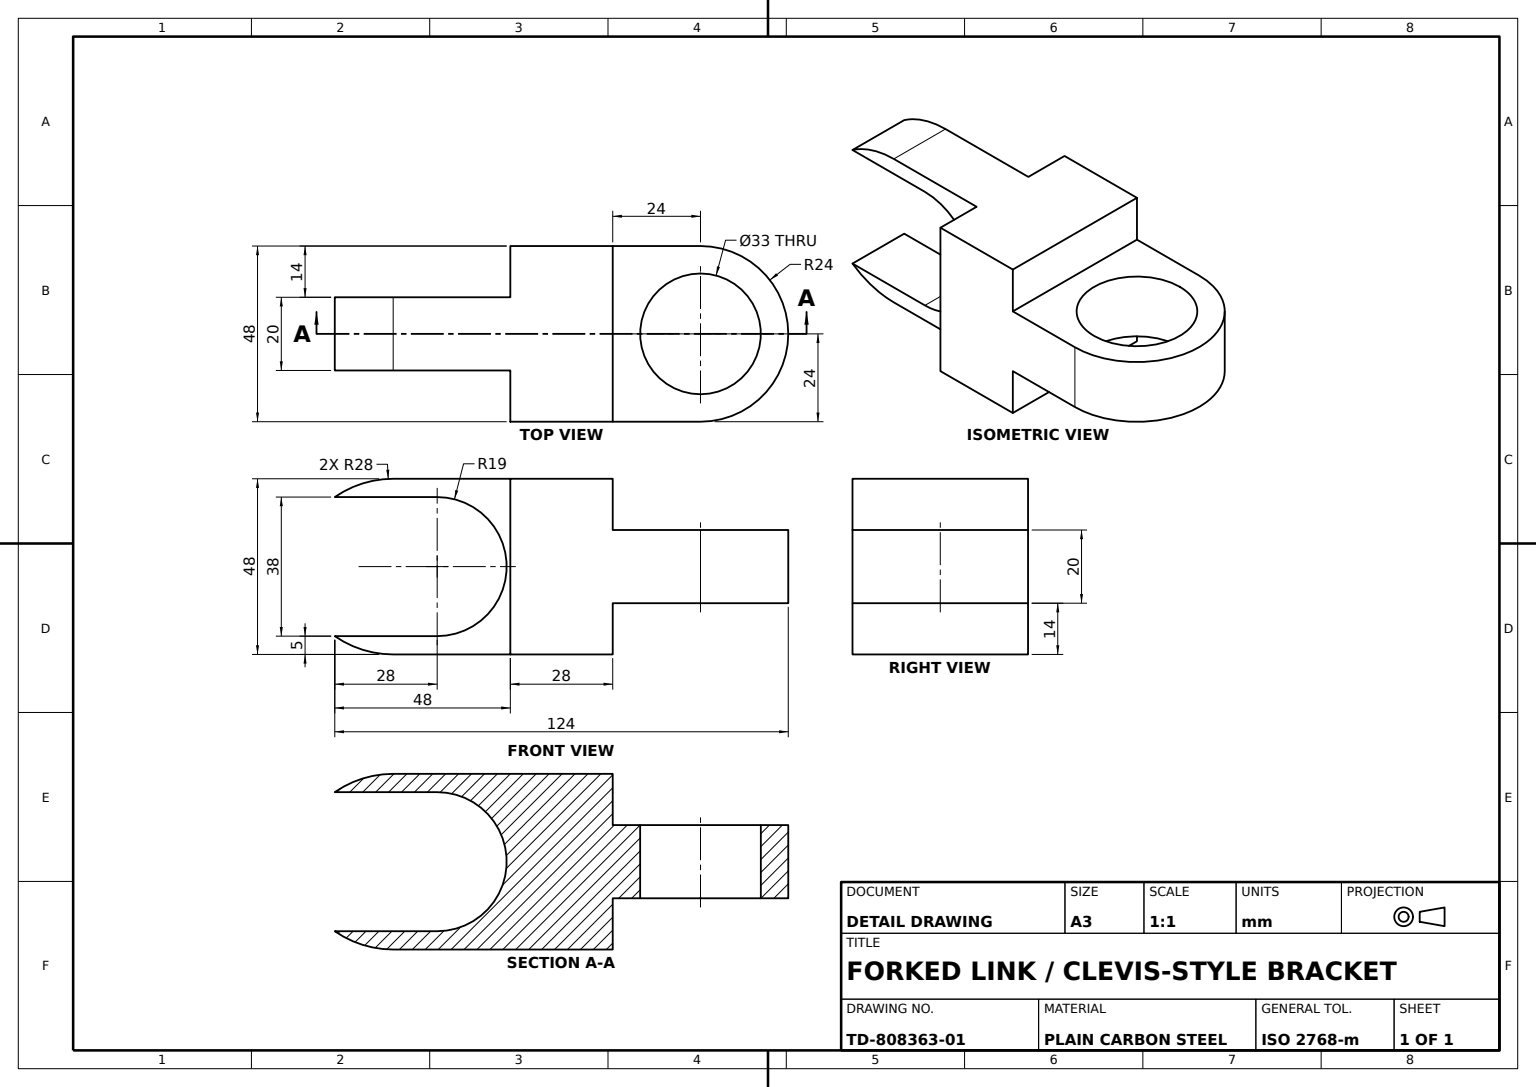
SolidWorks part; units mm, degrees
material "Plain Carbon Steel"
ref_plane "Front Plane" through (0, 0, 0) normal (0, 0, 1) x (1, 0, 0)
ref_plane "Top Plane" through (0, 0, 0) normal (0, 1, 0) x (1, 0, 0)
ref_plane "Right Plane" through (0, 0, 0) normal (1, 0, 0) x (0, 0, -1)
sketch "Base Block Sketch" plane through (0, 0, 0) normal (0, 0, 1) x (1, 0, 0)
  line L1 (0, 0) -> (28, 0)
  line L2 (0, 0) -> (0, -48)
  line L3 (0, -48) -> (28, -48)
  line L4 (28, 0) -> (28, -48)
  dimension "D1" = 48
  dimension "D2" = 28
extrude "Base Block" add sketch "Base Block Sketch" along normal mid plane 48
ref_plane "Fork Arms Plane" through (0, -24, 0) normal (0, 1, 0) x (1, 0, 0)
sketch "Fork Arms Sketch" plane through (0, -24, 0) normal (0, 1, 0) x (1, 0, 0)
  line L0 (28, 24) -> (28, -24) construction
  line L1 (28, -24) -> (76, -24) construction
  line L2 (76, -24) -> (76, 24) construction
  line L3 (76, 24) -> (28, 24) construction
  line L4 (28, 24) -> (28, -24)
  line L5 (28, -24) -> (52, -24)
  line L6 (52, -24) -> (52, 0)
  line L7 (52, 24) -> (28, 24)
  line L8 (0, 0) -> (52, 0) construction
  arc A0 (52, 24) -> (52, -24) centre (52, 0) cw
  dimension "D1" = 48
extrude "Fork Arms" add sketch "Fork Arms Sketch" along normal mid plane 20
sketch "Fork Arc Cut Sketch R33" plane through (0, -14, 0) normal (0, 1, 0) x (1, 0, 0)
  line L0 (0, 0) -> (62.8473, 0) construction
  circle A0 centre (52, 0) radius 16.5
  dimension "D1" = 33
extrude "Fork Arc Cut" cut sketch "Fork Arc Cut Sketch R33" against normal blind 20
sketch "Eye Lug Sketch" plane through (0, 0, 24) normal (0, 0, 1) x (1, 0, 0)
  line L0 (-20, 4.7884) -> (-20, -55.918) construction
  line L1 (0, 0) -> (0, -48) construction
  line L2 (0, -24) -> (-41.8079, -24) construction
  line L3 (0, 0) -> (-32.0313, 0)
  line L4 (-48, 0) -> (-48, -51.1042) construction
  line L5 (0, -48) -> (-32.0313, -48)
  line L6 (0, 0) -> (-41.8079, 0) construction
  line L7 (0, 0) -> (0, -48)
  line L8 (-20, -5) -> (-48, -5)
  line L10 (-20, -43) -> (-48, -43)
  arc A0 (-20, -43) -> (-20, -5) centre (-20, -24) ccw
  arc A1 (-48, -5) -> (-32.0313, 0) centre (-32.0313, -28) cw
  arc A2 (-48, -43) -> (-32.0313, -48) centre (-32.0313, -20) ccw
  dimension "D2" = 38
  dimension "D6" = 28
  dimension "D1" = 20
  dimension "D3" = 48
  dimension "D4" = 24
extrude "Eye Lug With Bore" add sketch "Eye Lug Sketch" along normal mid plane 20 from offset 24
